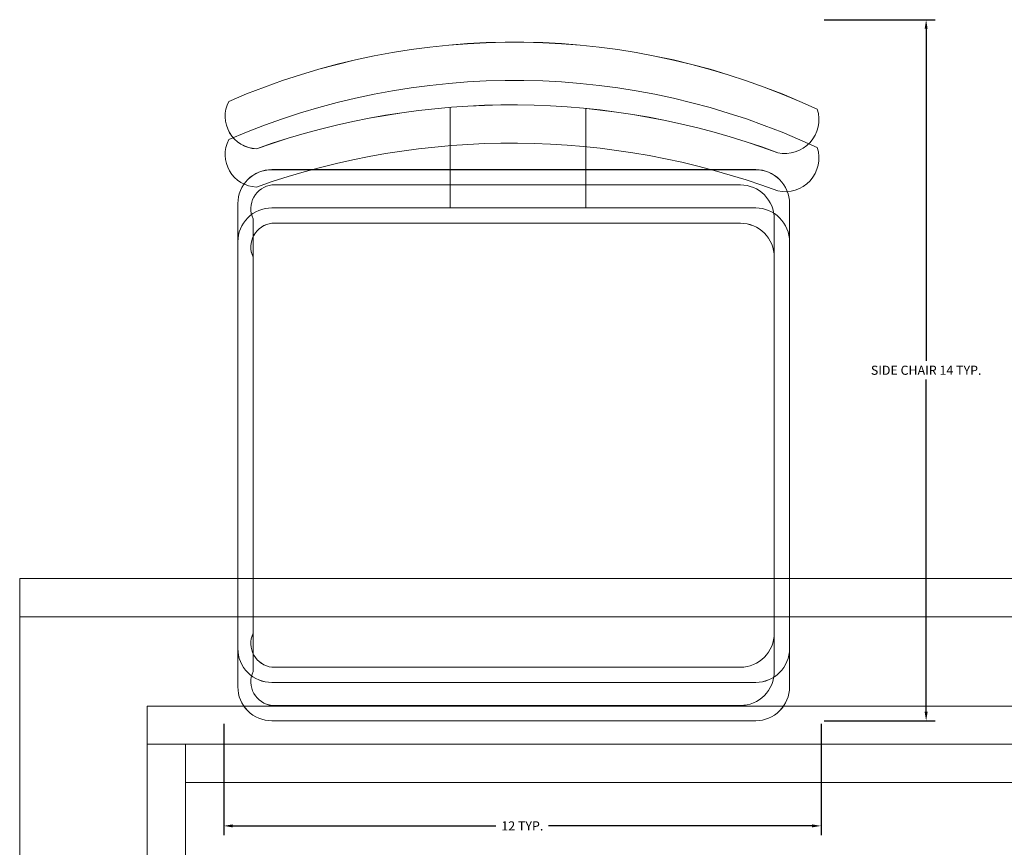
# Model space of a CAD drawing. Units: inches. Extents: x 1885 to 2748, y 783 to 2421.
# Tile 82 of 117: x 2137.01 to 2156.44, y 2095.3 to 2111.64. Entities that reach past the tile are written whole.
import ezdxf

# ---------------------------------------------------------------- set-up
doc = ezdxf.new("R2010")
doc.units = ezdxf.units.IN
doc.layers.add('A-ANNO-DIMS', color=2, linetype='Continuous', lineweight=18)
doc.layers.add('A-FURN', color=8, linetype='Continuous', lineweight=13)
doc.styles.get("Standard").update_dxf_attribs({"font": 'arial.ttf'})
doc.dimstyles.get("Standard").update_dxf_attribs({"dimtxt": 0.18, "dimasz": 0.18, "dimexe": 0.18, "dimexo": 0.0625, "dimgap": 0.09, "dimtad": 0, "dimtih": 1, "dimtoh": 1, "dimdec": 4, "dimzin": 0, "dimdsep": 46, "dimtxsty": 'Standard', "dimcen": 0.09, "dimadec": 0, "dimazin": 0, "dimtfac": 1, "dimtdec": 4, "dimtofl": 0, "dimtmove": 0, "dimatfit": 3, "dimfxl": 1, "dimtolj": 1, "dimtzin": 0, "dimarcsym": 0})

# ---------------------------------------------------------------- blocks, each defined once
blk = doc.blocks.new('TABLE-DINING-RECT')
for points in [[(-0.004, 23.421), (37.776, 23.421), (37.776, 0.754), (-0.004, 0.754)], [(-0.004, 23.421), (37.776, 23.421), (37.776, 0.753), (-0.004, 0.753)], [(-0.004, 22.666), (37.776, 22.666), (37.776, -0.002), (-0.004, -0.002)], [(-0.004, 22.665), (37.776, 22.665), (37.776, -0.002), (-0.004, -0.002)], [(2.515, 20.903), (35.257, 20.903), (35.257, 3.272), (2.515, 3.272)], [(2.515, 20.902), (35.257, 20.902), (35.257, 3.272), (2.515, 3.272)], [(2.515, 20.147), (35.257, 20.147), (35.257, 2.517), (2.515, 2.517)], [(2.515, 20.147), (35.257, 20.147), (35.257, 2.516), (2.515, 2.516)], [(3.27, 20.147), (34.501, 20.147), (34.501, 4.028), (3.27, 4.028)], [(3.27, 20.147), (34.501, 20.147), (34.501, 4.027), (3.27, 4.027)], [(3.27, 19.391), (34.501, 19.391), (34.501, 3.272), (3.27, 3.272)], [(3.27, 19.391), (34.501, 19.391), (34.501, 3.272), (3.27, 3.272)]]:
    blk.add_lwpolyline(points, close=True)
blk = doc.blocks.new('CHAIR-DINING-SIDE')
for points in [[(0.617, 11.293, -0.175809), (10.907, 11.215, 0.578392), (11.687, 12.072, 0.214524), (0.072, 12.228, 0.552014), (0.617, 11.293, -0.065079)], [(0.617, 11.292, -0.175809), (10.907, 11.214, 0.578392), (11.687, 12.071, 0.214524), (0.072, 12.227, 0.552014), (0.617, 11.292, -0.065079)], [(0.617, 10.537, -0.175809), (10.907, 10.459, 0.578392), (11.687, 11.316, 0.214524), (0.072, 11.472, 0.552014), (0.617, 10.537, -0.065079)], [(0.617, 10.537, -0.175809), (10.907, 10.459, 0.578392), (11.687, 11.316, 0.214524), (0.072, 11.472, 0.552014), (0.617, 10.537, -0.065079)], [(7.115, 10.88), (7.115, 12.088, -0.064759)], [(7.115, 10.879), (7.115, 12.087, -0.064759)], [(7.115, 10.124), (7.115, 11.332, -0.064759)], [(7.115, 10.124), (7.115, 11.332, -0.064759)], [(10.471, 10.88), (0.918, 10.88, 0.414214), (0.25, 10.211), (0.25, 1.428, 0.414214), (0.918, 0.759), (10.471, 0.759, 0.414214), (11.139, 1.428), (11.139, 10.211, 0.414214), (10.471, 10.88)], [(10.471, 10.879), (0.918, 10.879, 0.414214), (0.25, 10.211), (0.25, 1.427, 0.414214), (0.918, 0.759), (10.471, 0.759, 0.414214), (11.139, 1.427), (11.139, 10.211, 0.414214), (10.471, 10.879)], [(10.471, 10.124), (0.918, 10.124, 0.414214), (0.25, 9.456), (0.25, 0.672, 0.414214), (0.918, 0.004), (10.471, 0.004, 0.414214), (11.139, 0.672), (11.139, 9.456, 0.414214), (10.471, 10.124)], [(10.471, 10.124), (0.918, 10.124, 0.414214), (0.25, 9.455), (0.25, 0.672, 0.414214), (0.918, 0.003), (10.471, 0.003, 0.414214), (11.139, 0.672), (11.139, 9.455, 0.414214), (10.471, 10.124)]]:
    blk.add_lwpolyline(points, format="xyb")
for points in [[(4.441, 12.11), (4.441, 10.88)], [(4.441, 12.109), (4.441, 10.879)], [(4.441, 11.354), (4.441, 10.124)], [(4.441, 11.354), (4.441, 10.124)]]:
    blk.add_lwpolyline(points)
for points in [[(0.922, 10.578), (10.17, 10.578, -0.414214), (10.838, 9.91), (10.838, 1.729, -0.414214), (10.17, 1.06), (0.922, 1.06, -0.512069), (0.551, 1.729), (0.551, 9.91, -0.512069)], [(0.922, 10.578), (10.17, 10.578, -0.414214), (10.838, 9.91), (10.838, 1.728, -0.414214), (10.17, 1.06), (0.922, 1.06, -0.512069), (0.551, 1.728), (0.551, 9.91, -0.512069)], [(0.922, 9.823), (10.17, 9.823, -0.414214), (10.838, 9.155), (10.838, 0.973, -0.414214), (10.17, 0.305), (0.922, 0.305, -0.512069), (0.551, 0.973), (0.551, 9.155, -0.512069)], [(0.922, 9.822), (10.17, 9.822, -0.414214), (10.838, 9.154), (10.838, 0.973, -0.414214), (10.17, 0.304), (0.922, 0.304, -0.512069), (0.551, 0.973), (0.551, 9.154, -0.512069)]]:
    blk.add_lwpolyline(points, format="xyb", close=True)
blk = doc.blocks.new('*D37')
at = {"layer": 'A-ANNO-DIMS', "color": 0, "lineweight": -2, "transparency": 16777216}
for p, q in [((2152.888, 2111.638), (2155.081, 2111.638)), ((2154.901, 2111.458), (2154.901, 2104.903)), ((2154.901, 2097.982), (2154.901, 2104.537)), ((2152.888, 2097.802), (2155.081, 2097.802))]:
    blk.add_line(p, q, dxfattribs=at)
at = {"layer": 'A-ANNO-DIMS', "color": 0, "transparency": 16777216}
for points in [[(2154.871, 2111.458), (2154.931, 2111.458), (2154.901, 2111.638)], [(2154.871, 2097.982), (2154.931, 2097.982), (2154.901, 2097.802)]]:
    blk.add_solid(points, dxfattribs=at)
at = {"layer": 'Defpoints', "color": 0, "transparency": 16777216}
for p in [(2152.826, 2111.638), (2154.901, 2111.638), (2152.826, 2097.802)]:
    blk.add_point(p, dxfattribs=at)
at = {"layer": 'A-ANNO-DIMS', "color": 0, "transparency": 16777216, "insert": (2154.901, 2104.72), "char_height": 0.18, "attachment_point": 5}
blk.add_mtext('\\A1;SIDE CHAIR 14 TYP.', dxfattribs=at)
blk = doc.blocks.new('*D38')
at = {"layer": 'A-ANNO-DIMS', "color": 0, "lineweight": -2, "transparency": 16777216}
for p, q in [((2141.036, 2097.74), (2141.036, 2095.547)), ((2152.826, 2097.74), (2152.826, 2095.547)), ((2141.216, 2095.727), (2146.411, 2095.727)), ((2152.646, 2095.727), (2147.45, 2095.727))]:
    blk.add_line(p, q, dxfattribs=at)
at = {"layer": 'A-ANNO-DIMS', "color": 0, "transparency": 16777216}
for points in [[(2141.216, 2095.757), (2141.216, 2095.697), (2141.036, 2095.727)], [(2152.646, 2095.757), (2152.646, 2095.697), (2152.826, 2095.727)]]:
    blk.add_solid(points, dxfattribs=at)
at = {"layer": 'Defpoints', "color": 0, "transparency": 16777216}
for p in [(2141.036, 2097.802), (2152.826, 2097.802), (2152.826, 2095.727)]:
    blk.add_point(p, dxfattribs=at)
at = {"layer": 'A-ANNO-DIMS', "color": 0, "transparency": 16777216, "insert": (2146.931, 2095.727), "char_height": 0.18, "attachment_point": 5}
blk.add_mtext('\\A1;12 TYP.', dxfattribs=at)

msp = doc.modelspace()

# ---------------------------------------------------------------- block references
at = {"layer": 'A-FURN'}
for name, p in [('CHAIR-DINING-SIDE', (2141.066, 2097.799)), ('TABLE-DINING-RECT', (2137.014, 2077.19))]:
    msp.add_blockref(name, p, dxfattribs=at)

# ---------------------------------------------------------------- dimensions: what is measured, and where the dimension line sits
at = {"layer": 'A-ANNO-DIMS'}
dim = msp.add_linear_dim(base=(2154.901, 2111.638), p1=(2152.826, 2097.802), p2=(2152.826, 2111.638), angle=90, text='SIDE CHAIR <> TYP.', dimstyle='Standard', override={"dimdec": 0, "dimlfac": 1, "dimrnd": 0, "dimzin": 0, "dimdsep": 46, "dimlunit": 2}, dxfattribs=at)
dim.commit()
dim.dimension.update_dxf_attribs({"geometry": '*D37', "text_midpoint": (2154.901, 2104.72)})
dim = msp.add_linear_dim(base=(2152.826, 2095.727), p1=(2141.036, 2097.802), p2=(2152.826, 2097.802), text='<> TYP.', dimstyle='Standard', override={"dimdec": 0, "dimlfac": 1, "dimrnd": 0, "dimzin": 0, "dimdsep": 46, "dimlunit": 2}, dxfattribs=at)
dim.commit()
dim.dimension.update_dxf_attribs({"geometry": '*D38', "text_midpoint": (2146.931, 2095.727)})

doc.saveas('drawing.dxf')
